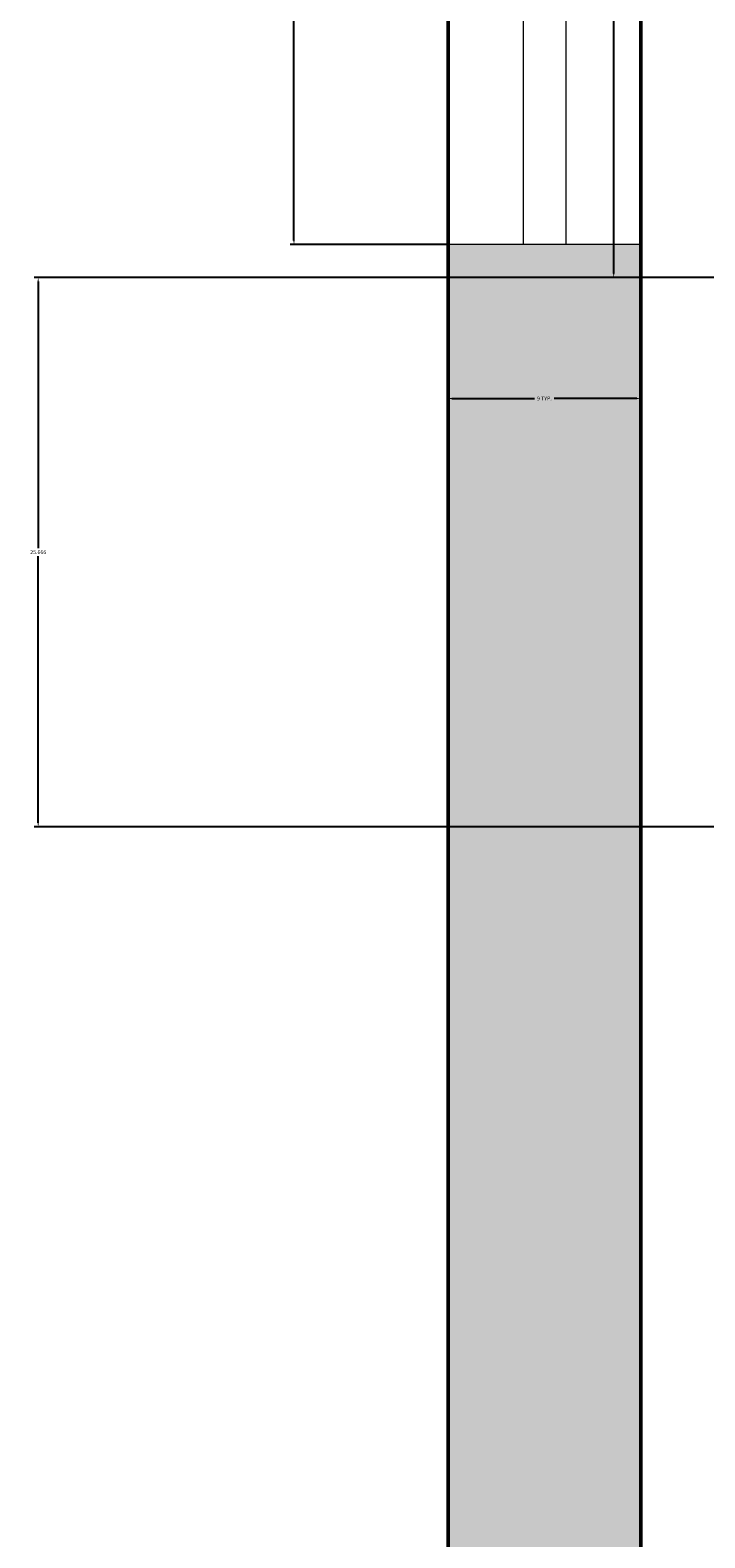
# Model space of a CAD drawing. Units: inches. Extents: x 2307 to 2544, y 2171 to 2540.
# Tile 4 of 52: x 2307 to 2339, y 2247 to 2317. Entities that reach past the tile are written whole.
import ezdxf

# ---------------------------------------------------------------- set-up
doc = ezdxf.new("R2010")
doc.units = ezdxf.units.IN
for name, color, linetype, lineweight in [('A-ANNO-DIMS', 2, 'Continuous', 18), ('A-GLAZ', 4, 'Continuous', 18), ('A-WALL', 7, 'Continuous', 50)]:
    doc.layers.add(name, color=color, linetype=linetype, lineweight=lineweight)
doc.layers.add('A-WALL-PATT', color=18, linetype='Continuous', lineweight=13, true_color=0x000000)
doc.styles.get("Standard").update_dxf_attribs({"font": 'arial.ttf'})
doc.dimstyles.get("Standard").update_dxf_attribs({"dimtxt": 0.18, "dimasz": 0.18, "dimexe": 0.18, "dimexo": 0.0625, "dimgap": 0.09, "dimtad": 0, "dimtih": 1, "dimtoh": 1, "dimdec": 4, "dimzin": 0, "dimdsep": 46, "dimtxsty": 'Standard', "dimcen": 0.09, "dimadec": 0, "dimazin": 0, "dimtfac": 1, "dimtdec": 4, "dimtofl": 0, "dimtmove": 0, "dimatfit": 3, "dimfxl": 1, "dimtolj": 1, "dimtzin": 0, "dimarcsym": 0})

# ---------------------------------------------------------------- blocks, each defined once
blk = doc.blocks.new('WIN-48IN')
for p, q in [((0, 5.5), (48, 5.5)), ((0, 3.5), (48, 3.5))]:
    blk.add_line(p, q)
for points in [[(0, 0), (0, 9)], [(48, 9), (48, 0)]]:
    blk.add_lwpolyline(points)
blk = doc.blocks.new('*D16')
at = {"layer": 'A-ANNO-DIMS', "color": 0, "lineweight": -2, "transparency": 16777216}
for p, q in [((2326.633, 2355.398), (2319.316, 2355.398)), ((2319.496, 2355.218), (2319.496, 2331.581)), ((2319.496, 2307.578), (2319.496, 2331.215)), ((2326.633, 2307.398), (2319.316, 2307.398))]:
    blk.add_line(p, q, dxfattribs=at)
at = {"layer": 'A-ANNO-DIMS', "color": 0, "transparency": 16777216}
for points in [[(2319.466, 2355.218), (2319.526, 2355.218), (2319.496, 2355.398)], [(2319.466, 2307.578), (2319.526, 2307.578), (2319.496, 2307.398)]]:
    blk.add_solid(points, dxfattribs=at)
at = {"layer": 'Defpoints', "color": 0, "transparency": 16777216}
for p in [(2326.696, 2355.398), (2319.496, 2307.398), (2326.696, 2307.398)]:
    blk.add_point(p, dxfattribs=at)
at = {"layer": 'A-ANNO-DIMS', "color": 0, "transparency": 16777216, "insert": (2319.496, 2331.398), "char_height": 0.18, "attachment_point": 5}
blk.add_mtext('\\A1;WINDOW 48 TYP.', dxfattribs=at)
blk = doc.blocks.new('*D17')
at = {"layer": 'A-ANNO-DIMS', "color": 0, "lineweight": -2, "transparency": 16777216}
for p, q in [((2326.696, 2307.336), (2326.696, 2300.018)), ((2335.696, 2307.336), (2335.696, 2300.018)), ((2326.876, 2300.198), (2330.738, 2300.198)), ((2335.516, 2300.198), (2331.654, 2300.198))]:
    blk.add_line(p, q, dxfattribs=at)
at = {"layer": 'A-ANNO-DIMS', "color": 0, "transparency": 16777216}
for points in [[(2326.876, 2300.228), (2326.876, 2300.168), (2326.696, 2300.198)], [(2335.516, 2300.228), (2335.516, 2300.168), (2335.696, 2300.198)]]:
    blk.add_solid(points, dxfattribs=at)
at = {"layer": 'Defpoints', "color": 0, "transparency": 16777216}
for p in [(2326.696, 2307.398), (2335.696, 2307.398), (2335.696, 2300.198)]:
    blk.add_point(p, dxfattribs=at)
at = {"layer": 'A-ANNO-DIMS', "color": 0, "transparency": 16777216, "insert": (2331.196, 2300.198), "char_height": 0.18, "attachment_point": 5}
blk.add_mtext('\\A1;9 TYP.', dxfattribs=at)
blk = doc.blocks.new('*D28')
at = {"layer": 'A-ANNO-DIMS', "color": 0, "lineweight": -2, "transparency": 16777216}
for p, q in [((2343.895, 2369.359), (2334.252, 2369.359)), ((2334.432, 2369.179), (2334.432, 2337.789)), ((2334.432, 2306.032), (2334.432, 2337.423)), ((2343.895, 2305.852), (2334.252, 2305.852))]:
    blk.add_line(p, q, dxfattribs=at)
at = {"layer": 'A-ANNO-DIMS', "color": 0, "transparency": 16777216}
for points in [[(2334.402, 2369.179), (2334.462, 2369.179), (2334.432, 2369.359)], [(2334.402, 2306.032), (2334.462, 2306.032), (2334.432, 2305.852)]]:
    blk.add_solid(points, dxfattribs=at)
at = {"layer": 'Defpoints', "color": 0, "transparency": 16777216}
for p in [(2343.958, 2369.359), (2334.432, 2305.852), (2343.958, 2305.852)]:
    blk.add_point(p, dxfattribs=at)
at = {"layer": 'A-ANNO-DIMS', "color": 0, "transparency": 16777216, "insert": (2334.432, 2337.606), "char_height": 0.18, "attachment_point": 5}
blk.add_mtext('\\A1;DINING SET 64', dxfattribs=at)
blk = doc.blocks.new('*D66')
at = {"layer": 'A-ANNO-DIMS', "color": 0, "lineweight": -2, "transparency": 16777216}
for p, q in [((2358.699, 2305.852), (2307.366, 2305.852)), ((2307.546, 2305.672), (2307.546, 2293.201)), ((2307.546, 2280.366), (2307.546, 2292.837)), ((2341.393, 2280.186), (2307.366, 2280.186))]:
    blk.add_line(p, q, dxfattribs=at)
at = {"layer": 'A-ANNO-DIMS', "color": 0, "transparency": 16777216}
for points in [[(2307.516, 2305.672), (2307.576, 2305.672), (2307.546, 2305.852)], [(2307.516, 2280.366), (2307.576, 2280.366), (2307.546, 2280.186)]]:
    blk.add_solid(points, dxfattribs=at)
at = {"layer": 'Defpoints', "color": 0, "transparency": 16777216}
for p in [(2307.546, 2305.852), (2358.761, 2305.852), (2341.456, 2280.186)]:
    blk.add_point(p, dxfattribs=at)
at = {"layer": 'A-ANNO-DIMS', "color": 0, "transparency": 16777216, "insert": (2307.546, 2293.019), "char_height": 0.18, "attachment_point": 5}
blk.add_mtext('\\A1;25.666', dxfattribs=at)

msp = doc.modelspace()

# ---------------------------------------------------------------- hatches: boundary and pattern name
at = {"layer": 'A-WALL-PATT'}
h = msp.add_hatch(color=256, dxfattribs=at)
h.dxf.hatch_style = 1
h.paths.add_polyline_path([(2433.6935, 2199.5096), (2415.6423, 2199.5096), (2415.6423, 2190.5096), (2433.7832, 2190.5096)], flags=17)
h.paths.add_polyline_path([(2367.6423, 2199.5096), (2335.6958, 2199.5096), (2335.6958, 2307.3983), (2326.6958, 2307.3983), (2326.6958, 2190.5096), (2367.6423, 2190.5096)])
h.paths.add_polyline_path([(2524.6958, 2520.5096), (2496.7832, 2520.5096), (2496.7832, 2515.5149), (2472.7832, 2515.5149), (2472.7832, 2520.5096), (2415.4028, 2520.5096), (2415.4028, 2511.5096), (2451.6958, 2511.5096), (2451.6958, 2439.5096), (2451.6958, 2391.5096), (2445.6958, 2391.5096), (2445.6958, 2387.5096), (2455.6958, 2387.5096), (2455.6958, 2435.5096), (2461.6958, 2435.5096), (2461.6958, 2439.5096), (2455.6958, 2439.5096), (2455.6958, 2511.5096), (2515.6958, 2511.5096), (2515.6958, 2439.5096), (2491.6958, 2439.5096), (2491.6958, 2435.5096), (2515.6958, 2435.5096), (2515.6958, 2319.5096), (2451.6958, 2319.5096), (2451.6958, 2281.5096), (2481.6958, 2281.5096), (2481.6958, 2225.5096), (2485.6958, 2225.5096), (2485.6958, 2285.5096), (2455.6958, 2285.5096), (2455.6958, 2315.5096), (2515.6958, 2315.5096), (2515.6958, 2199.5096), (2469.6952, 2199.5096), (2469.785, 2190.5096), (2524.6958, 2190.5096)])

# ---------------------------------------------------------------- linework, layer by layer
at = {"layer": 'A-WALL'}
msp.add_line((2335.6958, 2199.5096), (2335.6958, 2387.5096), dxfattribs=at)
msp.add_lwpolyline([(2433.7832, 2190.5096), (2326.6958, 2190.5096), (2326.6958, 2520.5096), (2524.6958, 2520.5096), (2524.6958, 2190.5096), (2469.785, 2190.5096)], dxfattribs=at)

# ---------------------------------------------------------------- block references
at = {"layer": 'A-GLAZ', "rotation": 270.0000000000004}
msp.add_blockref('WIN-48IN', (2326.6963, 2355.3986), dxfattribs=at)

# ---------------------------------------------------------------- dimensions: what is measured, and where the dimension line sits
at = {"layer": 'A-ANNO-DIMS'}
for base, p1, p2, text, picture, middle in [((2334.4318, 2305.8523), (2343.9578, 2369.3589), (2343.9578, 2305.8523), 'DINING SET <>', '*D28', (2334.4318, 2337.6056)), ((2319.4958, 2307.3983), (2326.6958, 2355.3983), (2326.6958, 2307.3983), 'WINDOW <> TYP.', '*D16', (2319.4958, 2331.3983))]:
    dim = msp.add_linear_dim(base=base, p1=p1, p2=p2, angle=270, text=text, dimstyle='Standard', override={"dimdec": 0, "dimlfac": 1, "dimrnd": 0, "dimzin": 0, "dimdsep": 46, "dimlunit": 2}, dxfattribs=at)
    dim.commit()
    dim.dimension.update_dxf_attribs({"geometry": picture, "text_midpoint": middle})
dim = msp.add_linear_dim(base=(2335.6958, 2300.1983), p1=(2326.6958, 2307.3983), p2=(2335.6958, 2307.3983), text='<> TYP.', dimstyle='Standard', override={"dimdec": 0, "dimlfac": 1, "dimrnd": 0, "dimzin": 0, "dimdsep": 46, "dimlunit": 2}, dxfattribs=at)
dim.commit()
dim.dimension.update_dxf_attribs({"geometry": '*D17', "text_midpoint": (2331.1958, 2300.1983)})
dim = msp.add_linear_dim(base=(2307.54584, 2305.85226), p1=(2341.45575, 2280.18577), p2=(2358.76101, 2305.85226), angle=90, dimstyle='Standard', override={"dimdec": 3, "dimlfac": 1, "dimrnd": 0, "dimzin": 0, "dimdsep": 46, "dimlunit": 2}, dxfattribs=at)
dim.commit()
dim.dimension.update_dxf_attribs({"geometry": '*D66', "text_midpoint": (2307.54584, 2293.01902)})

doc.saveas('drawing.dxf')
